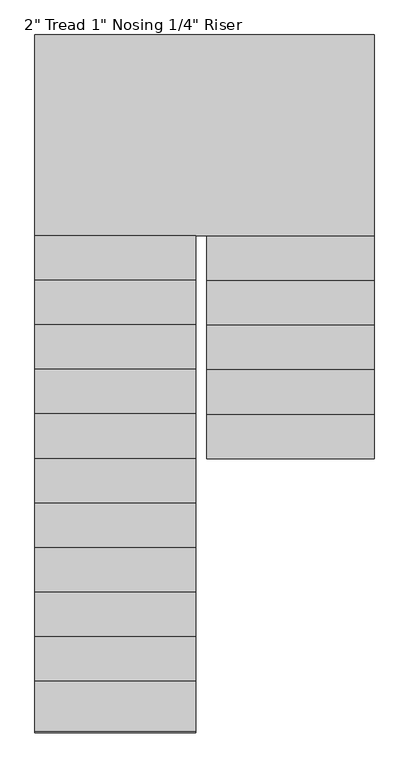
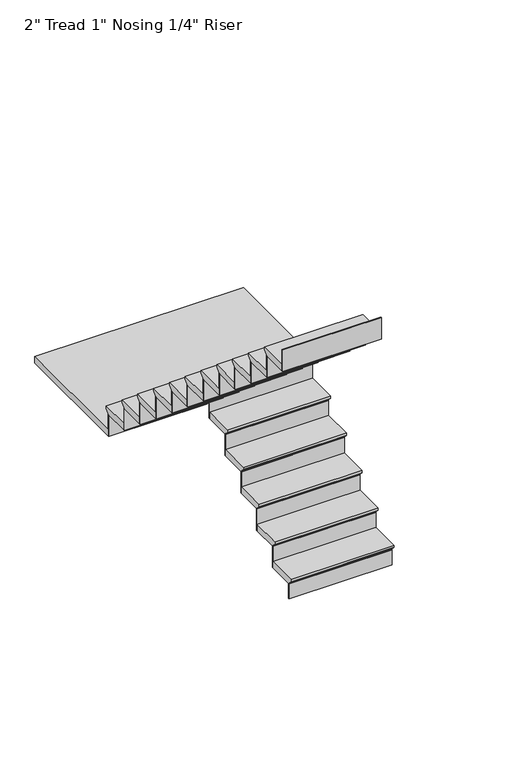
"""IFC4 building model written with IfcOpenShell, lengths in millimetres: stair flight geometry."""

from ifc_helpers import new_model, si_unit, origin, place, context, project, spatial, faceted_brep, source, transform, mapped, element, save


def stair_flight_f2d67c03(model_context):
    return source(origin(), model_context, "Body", "Brep", [
        faceted_brep([(-3749.597125, 2714.6319226, 21333.8833333), (-3749.597125, 2714.6319226, 21352.9333333), (-4512.2136682, 2714.6319226, 21352.9333333), (-4512.2136682, 2714.6319226, 21333.8833333), (-3749.597125, 2740.0319226, 21308.4833333), (-4512.2136682, 2740.0319226, 21308.4833333), (-3749.597125, 2943.2319226, 21352.9333333), (-4512.2136682, 2943.2319226, 21352.9333333), (-4512.2136682, 2740.0319226, 21302.1333333), (-4512.2136682, 2943.2319226, 21302.1333333), (-3749.597125, 2943.2319226, 21302.1333333), (-3749.597125, 2740.0319226, 21302.1333333)], [[[0, 1, 2, 3]], [[4, 0, 3, 5]], [[2, 1, 6, 7]], [[8, 9, 10, 11]], [[2, 7, 9, 8, 5, 3]], [[8, 11, 4, 5]], [[6, 1, 0, 4, 11, 10]], [[7, 6, 10, 9]]]),
        faceted_brep([(-3749.597125, 2740.0319226, 21302.1333333), (-3749.597125, 2740.0319226, 21183.6), (-3749.597125, 2746.3819226, 21183.6), (-3749.597125, 2746.3819226, 21302.1333333), (-4512.2136682, 2740.0319226, 21302.1333333), (-4512.2136682, 2746.3819226, 21302.1333333), (-4512.2136682, 2746.3819226, 21183.6), (-4512.2136682, 2740.0319226, 21183.6)], [[[0, 1, 2, 3]], [[4, 5, 6, 7]], [[1, 0, 4, 7]], [[2, 1, 7, 6]], [[3, 2, 6, 5]], [[0, 3, 5, 4]]]),
        faceted_brep([(-3749.597125, 2943.2319226, 21471.4666667), (-3749.597125, 2943.2319226, 21302.1333333), (-3749.597125, 2949.5819226, 21302.1333333), (-3749.597125, 2949.5819226, 21471.4666667), (-4512.2136682, 2943.2319226, 21471.4666667), (-4512.2136682, 2949.5819226, 21471.4666667), (-4512.2136682, 2949.5819226, 21302.1333333), (-4512.2136682, 2943.2319226, 21302.1333333)], [[[0, 1, 2, 3]], [[4, 5, 6, 7]], [[1, 0, 4, 7]], [[2, 1, 7, 6]], [[3, 2, 6, 5]], [[0, 3, 5, 4]]]),
        faceted_brep([(-4512.2136682, 2917.8319226, 21522.2666667), (-3749.597125, 2917.8319226, 21522.2666667), (-3749.597125, 3146.4319226, 21522.2666667), (-4512.2136682, 3146.4319226, 21522.2666667), (-4512.2136682, 2943.2319226, 21471.4666667), (-4512.2136682, 3146.4319226, 21471.4666667), (-3749.597125, 3146.4319226, 21471.4666667), (-3749.597125, 2943.2319226, 21471.4666667), (-4512.2136682, 2943.2319226, 21477.8166667), (-4512.2136682, 2917.8319226, 21503.2166667), (-3749.597125, 2943.2319226, 21477.8166667), (-3749.597125, 2917.8319226, 21503.2166667)], [[[0, 1, 2, 3]], [[4, 5, 6, 7]], [[0, 3, 5, 4, 8, 9]], [[4, 7, 10, 8]], [[2, 1, 11, 10, 7, 6]], [[3, 2, 6, 5]], [[11, 1, 0, 9]], [[10, 11, 9, 8]]]),
        faceted_brep([(-3749.597125, 3146.4319226, 21640.8), (-3749.597125, 3146.4319226, 21471.4666667), (-3749.597125, 3152.7819226, 21471.4666667), (-3749.597125, 3152.7819226, 21640.8), (-4512.2136682, 3146.4319226, 21640.8), (-4512.2136682, 3152.7819226, 21640.8), (-4512.2136682, 3152.7819226, 21471.4666667), (-4512.2136682, 3146.4319226, 21471.4666667)], [[[0, 1, 2, 3]], [[4, 5, 6, 7]], [[1, 0, 4, 7]], [[2, 1, 7, 6]], [[3, 2, 6, 5]], [[0, 3, 5, 4]]]),
        faceted_brep([(-4512.2136682, 3121.0319226, 21691.6), (-3749.597125, 3121.0319226, 21691.6), (-3749.597125, 3349.6319226, 21691.6), (-4512.2136682, 3349.6319226, 21691.6), (-4512.2136682, 3146.4319226, 21640.8), (-4512.2136682, 3349.6319226, 21640.8), (-3749.597125, 3349.6319226, 21640.8), (-3749.597125, 3146.4319226, 21640.8), (-4512.2136682, 3146.4319226, 21647.15), (-4512.2136682, 3121.0319226, 21672.55), (-3749.597125, 3146.4319226, 21647.15), (-3749.597125, 3121.0319226, 21672.55)], [[[0, 1, 2, 3]], [[4, 5, 6, 7]], [[0, 3, 5, 4, 8, 9]], [[4, 7, 10, 8]], [[2, 1, 11, 10, 7, 6]], [[3, 2, 6, 5]], [[11, 1, 0, 9]], [[10, 11, 9, 8]]]),
        faceted_brep([(-3749.597125, 3349.6319226, 21810.1333333), (-3749.597125, 3349.6319226, 21640.8), (-3749.597125, 3355.9819226, 21640.8), (-3749.597125, 3355.9819226, 21810.1333333), (-4512.2136682, 3349.6319226, 21810.1333333), (-4512.2136682, 3355.9819226, 21810.1333333), (-4512.2136682, 3355.9819226, 21640.8), (-4512.2136682, 3349.6319226, 21640.8)], [[[0, 1, 2, 3]], [[4, 5, 6, 7]], [[1, 0, 4, 7]], [[2, 1, 7, 6]], [[3, 2, 6, 5]], [[0, 3, 5, 4]]]),
        faceted_brep([(-4512.2136682, 3324.2319226, 21860.9333333), (-3749.597125, 3324.2319226, 21860.9333333), (-3749.597125, 3552.8319226, 21860.9333333), (-4512.2136682, 3552.8319226, 21860.9333333), (-4512.2136682, 3349.6319226, 21810.1333333), (-4512.2136682, 3552.8319226, 21810.1333333), (-3749.597125, 3552.8319226, 21810.1333333), (-3749.597125, 3349.6319226, 21810.1333333), (-4512.2136682, 3349.6319226, 21816.4833333), (-4512.2136682, 3324.2319226, 21841.8833333), (-3749.597125, 3349.6319226, 21816.4833333), (-3749.597125, 3324.2319226, 21841.8833333)], [[[0, 1, 2, 3]], [[4, 5, 6, 7]], [[0, 3, 5, 4, 8, 9]], [[4, 7, 10, 8]], [[2, 1, 11, 10, 7, 6]], [[3, 2, 6, 5]], [[11, 1, 0, 9]], [[10, 11, 9, 8]]]),
        faceted_brep([(-3749.597125, 3552.8319226, 21979.4666667), (-3749.597125, 3552.8319226, 21810.1333333), (-3749.597125, 3559.1819226, 21810.1333333), (-3749.597125, 3559.1819226, 21979.4666667), (-4512.2136682, 3552.8319226, 21979.4666667), (-4512.2136682, 3559.1819226, 21979.4666667), (-4512.2136682, 3559.1819226, 21810.1333333), (-4512.2136682, 3552.8319226, 21810.1333333)], [[[0, 1, 2, 3]], [[4, 5, 6, 7]], [[1, 0, 4, 7]], [[2, 1, 7, 6]], [[3, 2, 6, 5]], [[0, 3, 5, 4]]]),
        faceted_brep([(-4512.2136682, 3527.4319226, 22030.2666667), (-3749.597125, 3527.4319226, 22030.2666667), (-3749.597125, 3756.0319226, 22030.2666667), (-4512.2136682, 3756.0319226, 22030.2666667), (-4512.2136682, 3552.8319226, 21979.4666667), (-4512.2136682, 3756.0319226, 21979.4666667), (-3749.597125, 3756.0319226, 21979.4666667), (-3749.597125, 3552.8319226, 21979.4666667), (-4512.2136682, 3552.8319226, 21985.8166667), (-4512.2136682, 3527.4319226, 22011.2166667), (-3749.597125, 3552.8319226, 21985.8166667), (-3749.597125, 3527.4319226, 22011.2166667)], [[[0, 1, 2, 3]], [[4, 5, 6, 7]], [[0, 3, 5, 4, 8, 9]], [[4, 7, 10, 8]], [[2, 1, 11, 10, 7, 6]], [[3, 2, 6, 5]], [[11, 1, 0, 9]], [[10, 11, 9, 8]]]),
        faceted_brep([(-3749.597125, 3756.0319226, 22148.8), (-3749.597125, 3756.0319226, 21979.4666667), (-3749.597125, 3762.3819226, 21979.4666667), (-3749.597125, 3762.3819226, 22148.8), (-4512.2136682, 3756.0319226, 22148.8), (-4512.2136682, 3762.3819226, 22148.8), (-4512.2136682, 3762.3819226, 21979.4666667), (-4512.2136682, 3756.0319226, 21979.4666667)], [[[0, 1, 2, 3]], [[4, 5, 6, 7]], [[1, 0, 4, 7]], [[2, 1, 7, 6]], [[3, 2, 6, 5]], [[0, 3, 5, 4]]]),
        faceted_brep([(-4563.0136682, 3705.2319226, 22199.6), (-4563.0136682, 3730.6319226, 22199.6), (-3749.597125, 3730.6319226, 22199.6), (-3749.597125, 4645.0319226, 22199.6), (-5295.0246464, 4645.0319226, 22199.6), (-5295.0246464, 3705.2319226, 22199.6), (-4563.0136682, 3730.6319226, 22148.8), (-4563.0136682, 3705.2319226, 22148.8), (-5295.0246464, 3705.2319226, 22148.8), (-5295.0246464, 4645.0319226, 22148.8), (-3749.597125, 4645.0319226, 22148.8), (-3749.597125, 3756.0319226, 22148.8), (-4512.2136682, 3756.0319226, 22148.8), (-4512.2136682, 3730.6319226, 22148.8), (-4512.2136682, 3730.6319226, 22180.55), (-3749.597125, 3730.6319226, 22180.55), (-4512.2136682, 3756.0319226, 22155.15), (-3749.597125, 3756.0319226, 22155.15)], [[[0, 1, 2, 3, 4, 5]], [[6, 7, 8, 9, 10, 11, 12, 13]], [[1, 0, 7, 6]], [[2, 1, 6, 13, 14, 15]], [[13, 12, 16, 14]], [[12, 11, 17, 16]], [[3, 2, 15, 17, 11, 10]], [[4, 3, 10, 9]], [[5, 4, 9, 8]], [[0, 5, 8, 7]], [[17, 15, 14, 16]]]),
        faceted_brep([(-5295.0246464, 3705.2319226, 22318.1333333), (-5295.0246464, 3705.2319226, 22148.8), (-5295.0246464, 3698.8819226, 22148.8), (-5295.0246464, 3698.8819226, 22318.1333333), (-4563.0136682, 3705.2319226, 22318.1333333), (-4563.0136682, 3698.8819226, 22318.1333333), (-4563.0136682, 3698.8819226, 22148.8), (-4563.0136682, 3705.2319226, 22148.8)], [[[0, 1, 2, 3]], [[4, 5, 6, 7]], [[1, 0, 4, 7]], [[2, 1, 7, 6]], [[3, 2, 6, 5]], [[0, 3, 5, 4]]]),
        faceted_brep([(-4563.0136682, 3730.6319226, 22368.9333333), (-5295.0246464, 3730.6319226, 22368.9333333), (-5295.0246464, 3502.0319226, 22368.9333333), (-4563.0136682, 3502.0319226, 22368.9333333), (-4563.0136682, 3705.2319226, 22318.1333333), (-4563.0136682, 3502.0319226, 22318.1333333), (-5295.0246464, 3502.0319226, 22318.1333333), (-5295.0246464, 3705.2319226, 22318.1333333), (-4563.0136682, 3705.2319226, 22324.4833333), (-4563.0136682, 3730.6319226, 22349.8833333), (-5295.0246464, 3705.2319226, 22324.4833333), (-5295.0246464, 3730.6319226, 22349.8833333)], [[[0, 1, 2, 3]], [[4, 5, 6, 7]], [[0, 3, 5, 4, 8, 9]], [[4, 7, 10, 8]], [[2, 1, 11, 10, 7, 6]], [[3, 2, 6, 5]], [[11, 1, 0, 9]], [[10, 11, 9, 8]]]),
        faceted_brep([(-5295.0246464, 3502.0319226, 22487.4666667), (-5295.0246464, 3502.0319226, 22318.1333333), (-5295.0246464, 3495.6819226, 22318.1333333), (-5295.0246464, 3495.6819226, 22487.4666667), (-4563.0136682, 3502.0319226, 22487.4666667), (-4563.0136682, 3495.6819226, 22487.4666667), (-4563.0136682, 3495.6819226, 22318.1333333), (-4563.0136682, 3502.0319226, 22318.1333333)], [[[0, 1, 2, 3]], [[4, 5, 6, 7]], [[1, 0, 4, 7]], [[2, 1, 7, 6]], [[3, 2, 6, 5]], [[0, 3, 5, 4]]]),
        faceted_brep([(-4563.0136682, 3527.4319226, 22538.2666667), (-5295.0246464, 3527.4319226, 22538.2666667), (-5295.0246464, 3298.8319226, 22538.2666667), (-4563.0136682, 3298.8319226, 22538.2666667), (-4563.0136682, 3502.0319226, 22487.4666667), (-4563.0136682, 3298.8319226, 22487.4666667), (-5295.0246464, 3298.8319226, 22487.4666667), (-5295.0246464, 3502.0319226, 22487.4666667), (-4563.0136682, 3502.0319226, 22493.8166667), (-4563.0136682, 3527.4319226, 22519.2166667), (-5295.0246464, 3502.0319226, 22493.8166667), (-5295.0246464, 3527.4319226, 22519.2166667)], [[[0, 1, 2, 3]], [[4, 5, 6, 7]], [[0, 3, 5, 4, 8, 9]], [[4, 7, 10, 8]], [[2, 1, 11, 10, 7, 6]], [[3, 2, 6, 5]], [[11, 1, 0, 9]], [[10, 11, 9, 8]]]),
        faceted_brep([(-5295.0246464, 3298.8319226, 22656.8), (-5295.0246464, 3298.8319226, 22487.4666667), (-5295.0246464, 3292.4819226, 22487.4666667), (-5295.0246464, 3292.4819226, 22656.8), (-4563.0136682, 3298.8319226, 22656.8), (-4563.0136682, 3292.4819226, 22656.8), (-4563.0136682, 3292.4819226, 22487.4666667), (-4563.0136682, 3298.8319226, 22487.4666667)], [[[0, 1, 2, 3]], [[4, 5, 6, 7]], [[1, 0, 4, 7]], [[2, 1, 7, 6]], [[3, 2, 6, 5]], [[0, 3, 5, 4]]]),
        faceted_brep([(-4563.0136682, 3324.2319226, 22707.6), (-5295.0246464, 3324.2319226, 22707.6), (-5295.0246464, 3095.6319226, 22707.6), (-4563.0136682, 3095.6319226, 22707.6), (-4563.0136682, 3298.8319226, 22656.8), (-4563.0136682, 3095.6319226, 22656.8), (-5295.0246464, 3095.6319226, 22656.8), (-5295.0246464, 3298.8319226, 22656.8), (-4563.0136682, 3298.8319226, 22663.15), (-4563.0136682, 3324.2319226, 22688.55), (-5295.0246464, 3298.8319226, 22663.15), (-5295.0246464, 3324.2319226, 22688.55)], [[[0, 1, 2, 3]], [[4, 5, 6, 7]], [[0, 3, 5, 4, 8, 9]], [[4, 7, 10, 8]], [[2, 1, 11, 10, 7, 6]], [[3, 2, 6, 5]], [[11, 1, 0, 9]], [[10, 11, 9, 8]]]),
        faceted_brep([(-5295.0246464, 3095.6319226, 22826.1333333), (-5295.0246464, 3095.6319226, 22656.8), (-5295.0246464, 3089.2819226, 22656.8), (-5295.0246464, 3089.2819226, 22826.1333333), (-4563.0136682, 3095.6319226, 22826.1333333), (-4563.0136682, 3089.2819226, 22826.1333333), (-4563.0136682, 3089.2819226, 22656.8), (-4563.0136682, 3095.6319226, 22656.8)], [[[0, 1, 2, 3]], [[4, 5, 6, 7]], [[1, 0, 4, 7]], [[2, 1, 7, 6]], [[3, 2, 6, 5]], [[0, 3, 5, 4]]]),
        faceted_brep([(-4563.0136682, 3121.0319226, 22876.9333333), (-5295.0246464, 3121.0319226, 22876.9333333), (-5295.0246464, 2892.4319226, 22876.9333333), (-4563.0136682, 2892.4319226, 22876.9333333), (-4563.0136682, 3095.6319226, 22826.1333333), (-4563.0136682, 2892.4319226, 22826.1333333), (-5295.0246464, 2892.4319226, 22826.1333333), (-5295.0246464, 3095.6319226, 22826.1333333), (-4563.0136682, 3095.6319226, 22832.4833333), (-4563.0136682, 3121.0319226, 22857.8833333), (-5295.0246464, 3095.6319226, 22832.4833333), (-5295.0246464, 3121.0319226, 22857.8833333)], [[[0, 1, 2, 3]], [[4, 5, 6, 7]], [[0, 3, 5, 4, 8, 9]], [[4, 7, 10, 8]], [[2, 1, 11, 10, 7, 6]], [[3, 2, 6, 5]], [[11, 1, 0, 9]], [[10, 11, 9, 8]]]),
        faceted_brep([(-5295.0246464, 2892.4319226, 22995.4666667), (-5295.0246464, 2892.4319226, 22826.1333333), (-5295.0246464, 2886.0819226, 22826.1333333), (-5295.0246464, 2886.0819226, 22995.4666667), (-4563.0136682, 2892.4319226, 22995.4666667), (-4563.0136682, 2886.0819226, 22995.4666667), (-4563.0136682, 2886.0819226, 22826.1333333), (-4563.0136682, 2892.4319226, 22826.1333333)], [[[0, 1, 2, 3]], [[4, 5, 6, 7]], [[1, 0, 4, 7]], [[2, 1, 7, 6]], [[3, 2, 6, 5]], [[0, 3, 5, 4]]]),
        faceted_brep([(-4563.0136682, 2917.8319226, 23046.2666667), (-5295.0246464, 2917.8319226, 23046.2666667), (-5295.0246464, 2689.2319226, 23046.2666667), (-4563.0136682, 2689.2319226, 23046.2666667), (-4563.0136682, 2892.4319226, 22995.4666667), (-4563.0136682, 2689.2319226, 22995.4666667), (-5295.0246464, 2689.2319226, 22995.4666667), (-5295.0246464, 2892.4319226, 22995.4666667), (-4563.0136682, 2892.4319226, 23001.8166667), (-4563.0136682, 2917.8319226, 23027.2166667), (-5295.0246464, 2892.4319226, 23001.8166667), (-5295.0246464, 2917.8319226, 23027.2166667)], [[[0, 1, 2, 3]], [[4, 5, 6, 7]], [[0, 3, 5, 4, 8, 9]], [[4, 7, 10, 8]], [[2, 1, 11, 10, 7, 6]], [[3, 2, 6, 5]], [[11, 1, 0, 9]], [[10, 11, 9, 8]]]),
        faceted_brep([(-5295.0246464, 2689.2319226, 23164.8), (-5295.0246464, 2689.2319226, 22995.4666667), (-5295.0246464, 2682.8819226, 22995.4666667), (-5295.0246464, 2682.8819226, 23164.8), (-4563.0136682, 2689.2319226, 23164.8), (-4563.0136682, 2682.8819226, 23164.8), (-4563.0136682, 2682.8819226, 22995.4666667), (-4563.0136682, 2689.2319226, 22995.4666667)], [[[0, 1, 2, 3]], [[4, 5, 6, 7]], [[1, 0, 4, 7]], [[2, 1, 7, 6]], [[3, 2, 6, 5]], [[0, 3, 5, 4]]]),
        faceted_brep([(-4563.0136682, 2714.6319226, 23215.6), (-5295.0246464, 2714.6319226, 23215.6), (-5295.0246464, 2486.0319226, 23215.6), (-4563.0136682, 2486.0319226, 23215.6), (-4563.0136682, 2689.2319226, 23164.8), (-4563.0136682, 2486.0319226, 23164.8), (-5295.0246464, 2486.0319226, 23164.8), (-5295.0246464, 2689.2319226, 23164.8), (-4563.0136682, 2689.2319226, 23171.15), (-4563.0136682, 2714.6319226, 23196.55), (-5295.0246464, 2689.2319226, 23171.15), (-5295.0246464, 2714.6319226, 23196.55)], [[[0, 1, 2, 3]], [[4, 5, 6, 7]], [[0, 3, 5, 4, 8, 9]], [[4, 7, 10, 8]], [[2, 1, 11, 10, 7, 6]], [[3, 2, 6, 5]], [[11, 1, 0, 9]], [[10, 11, 9, 8]]]),
        faceted_brep([(-5295.0246464, 2486.0319226, 23334.1333333), (-5295.0246464, 2486.0319226, 23164.8), (-5295.0246464, 2479.6819226, 23164.8), (-5295.0246464, 2479.6819226, 23334.1333333), (-4563.0136682, 2486.0319226, 23334.1333333), (-4563.0136682, 2479.6819226, 23334.1333333), (-4563.0136682, 2479.6819226, 23164.8), (-4563.0136682, 2486.0319226, 23164.8)], [[[0, 1, 2, 3]], [[4, 5, 6, 7]], [[1, 0, 4, 7]], [[2, 1, 7, 6]], [[3, 2, 6, 5]], [[0, 3, 5, 4]]]),
        faceted_brep([(-4563.0136682, 2511.4319226, 23384.9333333), (-5295.0246464, 2511.4319226, 23384.9333333), (-5295.0246464, 2282.8319226, 23384.9333333), (-4563.0136682, 2282.8319226, 23384.9333333), (-4563.0136682, 2486.0319226, 23334.1333333), (-4563.0136682, 2282.8319226, 23334.1333333), (-5295.0246464, 2282.8319226, 23334.1333333), (-5295.0246464, 2486.0319226, 23334.1333333), (-4563.0136682, 2486.0319226, 23340.4833333), (-4563.0136682, 2511.4319226, 23365.8833333), (-5295.0246464, 2486.0319226, 23340.4833333), (-5295.0246464, 2511.4319226, 23365.8833333)], [[[0, 1, 2, 3]], [[4, 5, 6, 7]], [[0, 3, 5, 4, 8, 9]], [[4, 7, 10, 8]], [[2, 1, 11, 10, 7, 6]], [[3, 2, 6, 5]], [[11, 1, 0, 9]], [[10, 11, 9, 8]]]),
        faceted_brep([(-5295.0246464, 2282.8319226, 23503.4666667), (-5295.0246464, 2282.8319226, 23334.1333333), (-5295.0246464, 2276.4819226, 23334.1333333), (-5295.0246464, 2276.4819226, 23503.4666667), (-4563.0136682, 2282.8319226, 23503.4666667), (-4563.0136682, 2276.4819226, 23503.4666667), (-4563.0136682, 2276.4819226, 23334.1333333), (-4563.0136682, 2282.8319226, 23334.1333333)], [[[0, 1, 2, 3]], [[4, 5, 6, 7]], [[1, 0, 4, 7]], [[2, 1, 7, 6]], [[3, 2, 6, 5]], [[0, 3, 5, 4]]]),
        faceted_brep([(-4563.0136682, 2308.2319226, 23554.2666667), (-5295.0246464, 2308.2319226, 23554.2666667), (-5295.0246464, 2079.6319226, 23554.2666667), (-4563.0136682, 2079.6319226, 23554.2666667), (-4563.0136682, 2282.8319226, 23503.4666667), (-4563.0136682, 2079.6319226, 23503.4666667), (-5295.0246464, 2079.6319226, 23503.4666667), (-5295.0246464, 2282.8319226, 23503.4666667), (-4563.0136682, 2282.8319226, 23509.8166667), (-4563.0136682, 2308.2319226, 23535.2166667), (-5295.0246464, 2282.8319226, 23509.8166667), (-5295.0246464, 2308.2319226, 23535.2166667)], [[[0, 1, 2, 3]], [[4, 5, 6, 7]], [[0, 3, 5, 4, 8, 9]], [[4, 7, 10, 8]], [[2, 1, 11, 10, 7, 6]], [[3, 2, 6, 5]], [[11, 1, 0, 9]], [[10, 11, 9, 8]]]),
        faceted_brep([(-5295.0246464, 2079.6319226, 23672.8), (-5295.0246464, 2079.6319226, 23503.4666667), (-5295.0246464, 2073.2819226, 23503.4666667), (-5295.0246464, 2073.2819226, 23672.8), (-4563.0136682, 2079.6319226, 23672.8), (-4563.0136682, 2073.2819226, 23672.8), (-4563.0136682, 2073.2819226, 23503.4666667), (-4563.0136682, 2079.6319226, 23503.4666667)], [[[0, 1, 2, 3]], [[4, 5, 6, 7]], [[1, 0, 4, 7]], [[2, 1, 7, 6]], [[3, 2, 6, 5]], [[0, 3, 5, 4]]]),
        faceted_brep([(-4563.0136682, 2105.0319226, 23723.6), (-5295.0246464, 2105.0319226, 23723.6), (-5295.0246464, 1876.4319226, 23723.6), (-4563.0136682, 1876.4319226, 23723.6), (-4563.0136682, 2079.6319226, 23672.8), (-4563.0136682, 1876.4319226, 23672.8), (-5295.0246464, 1876.4319226, 23672.8), (-5295.0246464, 2079.6319226, 23672.8), (-4563.0136682, 2079.6319226, 23679.15), (-4563.0136682, 2105.0319226, 23704.55), (-5295.0246464, 2079.6319226, 23679.15), (-5295.0246464, 2105.0319226, 23704.55)], [[[0, 1, 2, 3]], [[4, 5, 6, 7]], [[0, 3, 5, 4, 8, 9]], [[4, 7, 10, 8]], [[2, 1, 11, 10, 7, 6]], [[3, 2, 6, 5]], [[11, 1, 0, 9]], [[10, 11, 9, 8]]]),
        faceted_brep([(-5295.0246464, 1876.4319226, 23842.1333333), (-5295.0246464, 1876.4319226, 23672.8), (-5295.0246464, 1870.0819226, 23672.8), (-5295.0246464, 1870.0819226, 23842.1333333), (-4563.0136682, 1876.4319226, 23842.1333333), (-4563.0136682, 1870.0819226, 23842.1333333), (-4563.0136682, 1870.0819226, 23672.8), (-4563.0136682, 1876.4319226, 23672.8)], [[[0, 1, 2, 3]], [[4, 5, 6, 7]], [[1, 0, 4, 7]], [[2, 1, 7, 6]], [[3, 2, 6, 5]], [[0, 3, 5, 4]]]),
        faceted_brep([(-4563.0136682, 1901.8319226, 23892.9333333), (-5295.0246464, 1901.8319226, 23892.9333333), (-5295.0246464, 1673.2319226, 23892.9333333), (-4563.0136682, 1673.2319226, 23892.9333333), (-4563.0136682, 1876.4319226, 23842.1333333), (-4563.0136682, 1673.2319226, 23842.1333333), (-5295.0246464, 1673.2319226, 23842.1333333), (-5295.0246464, 1876.4319226, 23842.1333333), (-4563.0136682, 1876.4319226, 23848.4833333), (-4563.0136682, 1901.8319226, 23873.8833333), (-5295.0246464, 1876.4319226, 23848.4833333), (-5295.0246464, 1901.8319226, 23873.8833333)], [[[0, 1, 2, 3]], [[4, 5, 6, 7]], [[0, 3, 5, 4, 8, 9]], [[4, 7, 10, 8]], [[2, 1, 11, 10, 7, 6]], [[3, 2, 6, 5]], [[11, 1, 0, 9]], [[10, 11, 9, 8]]]),
        faceted_brep([(-5295.0246464, 1673.2319226, 24011.4666667), (-5295.0246464, 1673.2319226, 23842.1333333), (-5295.0246464, 1666.8819226, 23842.1333333), (-5295.0246464, 1666.8819226, 24011.4666667), (-4563.0136682, 1673.2319226, 24011.4666667), (-4563.0136682, 1666.8819226, 24011.4666667), (-4563.0136682, 1666.8819226, 23842.1333333), (-4563.0136682, 1673.2319226, 23842.1333333)], [[[0, 1, 2, 3]], [[4, 5, 6, 7]], [[1, 0, 4, 7]], [[2, 1, 7, 6]], [[3, 2, 6, 5]], [[0, 3, 5, 4]]]),
        faceted_brep([(-4563.0136682, 1698.6319226, 24062.2666667), (-5295.0246464, 1698.6319226, 24062.2666667), (-5295.0246464, 1470.0319226, 24062.2666667), (-4563.0136682, 1470.0319226, 24062.2666667), (-4563.0136682, 1673.2319226, 24011.4666667), (-4563.0136682, 1470.0319226, 24011.4666667), (-5295.0246464, 1470.0319226, 24011.4666667), (-5295.0246464, 1673.2319226, 24011.4666667), (-4563.0136682, 1673.2319226, 24017.8166667), (-4563.0136682, 1698.6319226, 24043.2166667), (-5295.0246464, 1673.2319226, 24017.8166667), (-5295.0246464, 1698.6319226, 24043.2166667)], [[[0, 1, 2, 3]], [[4, 5, 6, 7]], [[0, 3, 5, 4, 8, 9]], [[4, 7, 10, 8]], [[2, 1, 11, 10, 7, 6]], [[3, 2, 6, 5]], [[11, 1, 0, 9]], [[10, 11, 9, 8]]]),
        faceted_brep([(-5295.0246464, 1470.0319226, 24180.8), (-5295.0246464, 1470.0319226, 24011.4666667), (-5295.0246464, 1463.6819226, 24011.4666667), (-5295.0246464, 1463.6819226, 24180.8), (-4563.0136682, 1470.0319226, 24180.8), (-4563.0136682, 1463.6819226, 24180.8), (-4563.0136682, 1463.6819226, 24011.4666667), (-4563.0136682, 1470.0319226, 24011.4666667)], [[[0, 1, 2, 3]], [[4, 5, 6, 7]], [[1, 0, 4, 7]], [[2, 1, 7, 6]], [[3, 2, 6, 5]], [[0, 3, 5, 4]]]),
    ])


if __name__ == "__main__":
    model = new_model("IFC4")
    model_context = context("Model", 3, world=origin())
    ifc_project = project(units=[si_unit("LENGTHUNIT", "METRE", prefix="MILLI")], contexts=[model_context])
    site = spatial("IfcSite", under=ifc_project)
    building = spatial("IfcBuilding", under=site)
    placement = place(None, origin())
    stair_flight_shape = stair_flight_f2d67c03(model_context)
    element("IfcStairFlight", 1, ObjectType="2\" Tread 1\" Nosing 1/4\" Riser", at=placement, inside=building, context=model_context, shape_type="MappedRepresentation", body=[
        mapped(stair_flight_shape, transform((0.0, 0.0, 0.0), x_axis=(1.0, 0.0, 0.0), y_axis=(0.0, 1.0, 0.0), z_axis=(0.0, 0.0, 1.0))),
    ])
    save(model, "model.ifc")
